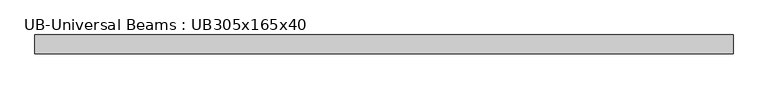
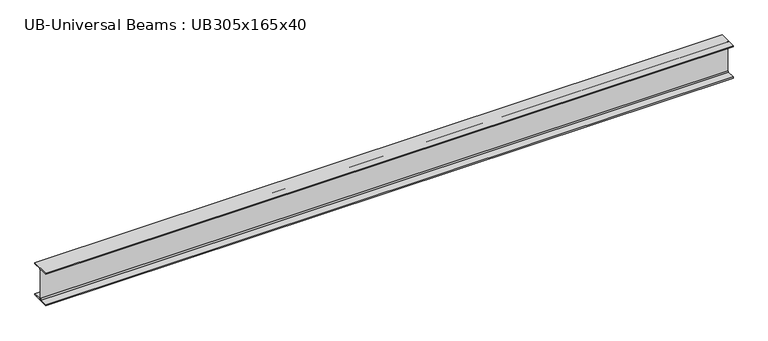
"""IFC4 building model written with IfcOpenShell, lengths in millimetres: beam geometry, UB-Universal Beams : UB305x165x40."""

from ifc_helpers import new_model, si_unit, point, frame, frame_2d, origin, place, context, project, spatial, polyline, circle_curve, trimmed, segment, composite_curve, outline, extrude, source, transform, mapped, element, save


def ub_universal_beams_ub305x165x40_f918ae41(model_context):
    return source(origin(), model_context, "Body", "SweptSolid", [
        extrude(outline(composite_curve([segment(polyline([(82.5, -141.5), (82.5, -151.7), (-82.5, -151.7), (-82.5, -141.5), (-11.9, -141.5)]), True, "CONTINUOUS"), segment(trimmed(circle_curve(frame_2d((-11.9, -132.6)), 8.9), [point((-11.9, -141.5))], [point((-3.0, -132.6))], True, "CARTESIAN"), True, "CONTINUOUS"), segment(polyline([(-3.0, -132.6), (-3.0, 132.6)]), True, "CONTINUOUS"), segment(trimmed(circle_curve(frame_2d((-11.9, 132.6)), 8.9), [point((-3.0, 132.6))], [point((-11.9, 141.5))], True, "CARTESIAN"), True, "CONTINUOUS"), segment(polyline([(-11.9, 141.5), (-82.5, 141.5), (-82.5, 151.7), (82.5, 151.7), (82.5, 141.5), (11.9, 141.5)]), True, "CONTINUOUS"), segment(trimmed(circle_curve(frame_2d((11.9, 132.6)), 8.9), [point((11.9, 141.5))], [point((3.0, 132.6))], True, "CARTESIAN"), True, "CONTINUOUS"), segment(polyline([(3.0, 132.6), (3.0, -132.6)]), True, "CONTINUOUS"), segment(trimmed(circle_curve(frame_2d((11.9, -132.6)), 8.9), [point((3.0, -132.6))], [point((11.9, -141.5))], True, "CARTESIAN"), True, "CONTINUOUS"), segment(polyline([(11.9, -141.5), (82.5, -141.5)]), True, "CONTINUOUS")], self_intersect=False)), frame((-3130.5, 0.0, 0.0), z_axis=(1.0, 0.0, 0.0), x_axis=(0.0, 1.0, 0.0)), (0.0, 0.0, 1.0), 6083.3),
    ])


if __name__ == "__main__":
    model = new_model("IFC4")
    model_context = context("Model", 3, world=origin())
    ifc_project = project(units=[si_unit("LENGTHUNIT", "METRE", prefix="MILLI")], contexts=[model_context])
    site = spatial("IfcSite", under=ifc_project)
    building = spatial("IfcBuilding", under=site)
    placement = place(None, origin())
    ub_universal_beams_ub305x165x40_shape = ub_universal_beams_ub305x165x40_f918ae41(model_context)
    element("IfcBeam", 1, ObjectType="UB-Universal Beams : UB305x165x40", at=placement, inside=building, context=model_context, shape_type="MappedRepresentation", body=[
        mapped(ub_universal_beams_ub305x165x40_shape, transform((0.0, 0.0, 0.0), x_axis=(1.0, 0.0, 0.0), y_axis=(0.0, 1.0, 0.0), z_axis=(0.0, 0.0, 1.0))),
    ])
    save(model, "model.ifc")

# Revit data of these elements
# Type "UB-Universal Beams : UB305x165x40"
#   Section Name Key = "UB305X165X40"
#   Width = 16.5 cm
#   Web Thickness = 0.6 cm
#   Web Fillet = 0.89 cm
#   Warping Constant = 164000.0 cm⁶
#   Torsional Moment of Inertia = 14.70 cm⁴
#   Section Area = 51.3 cm²
#   Plastic Modulus weak axis = 142.0 cm³
#   Plastic Modulus strong axis = 623.0 cm³
#   Nominal Weight = 40.2999 kgf/m
#   Moment of Inertia weak axis = 764.00 cm⁴
#   Moment of Inertia strong axis = 8503.00 cm⁴
#   Height = 30.34 cm
#   Flange Thickness = 1.02 cm
#   Elastic Modulus weak axis = 92.6 cm³
#   Elastic Modulus strong axis = 560.0 cm³
#   Centroid Vertical = 15.17 cm
#   Centroid Horizontal = 8.25 cm
#   Bolt Spacing = 9.0 cm
#   Length [instance default] = 1500 mm
#   Structural Material [instance default] = Metal - Steel 43-275
#   Type Comments = ""
#   Assembly Code = ""
# Element 1 (IfcBeam, "UB-Universal Beams : UB305x165x40")
#   Materials on its faces: "Metal - Steel 43-275"
# Materials
#   "Metal - Steel 43-275": class "Metal", colour RGB 247 247 247, transparency 0, Cost = 0
